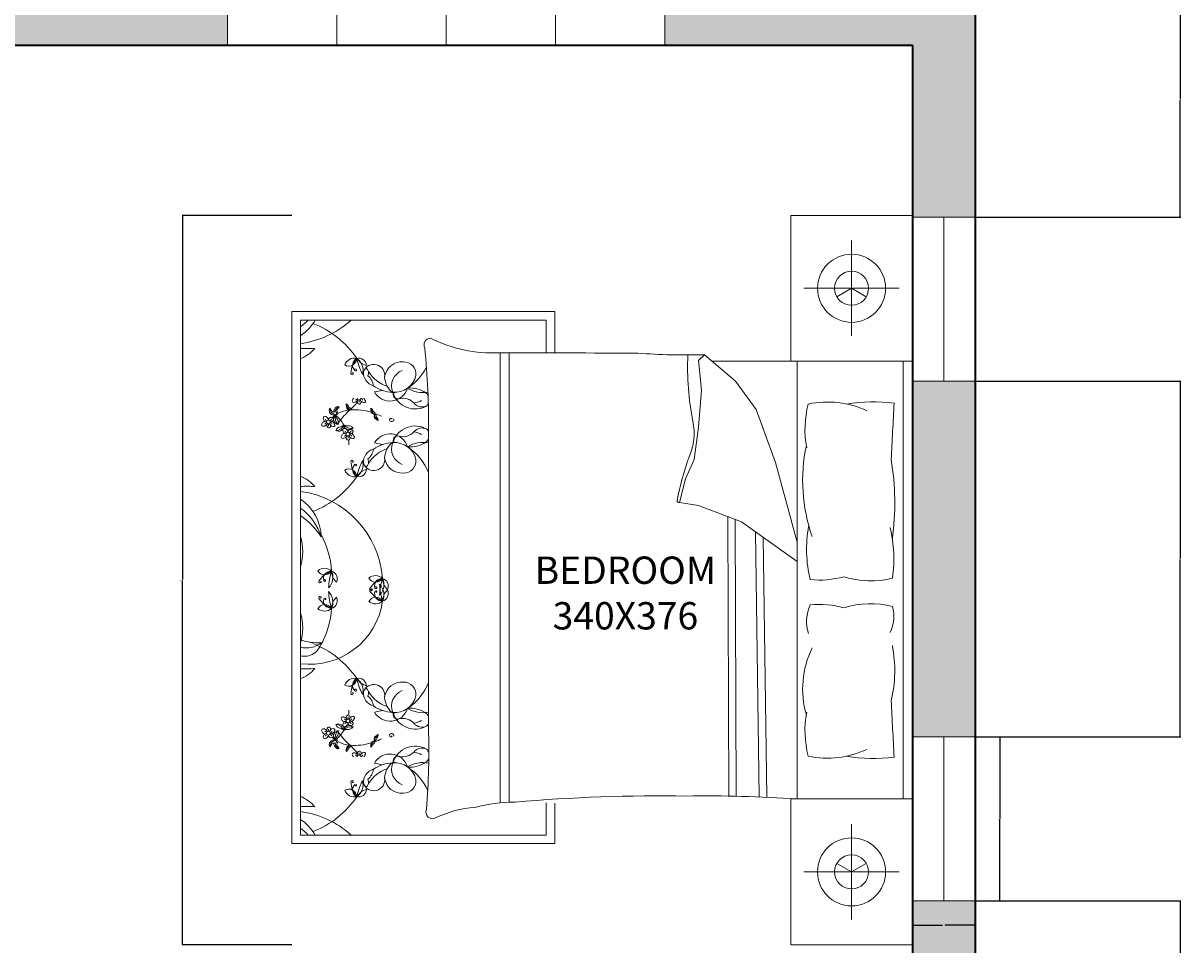
# Model space of a CAD drawing. Units: centimetres. Extents: x 2178 to 3635, y 1064 to 2635.
# Tile 8 of 9: x 3211 to 3635, y 1974 to 2312. Entities that reach past the tile are written whole.
import ezdxf

# ---------------------------------------------------------------- set-up
doc = ezdxf.new("R2010")
doc.units = ezdxf.units.CM
for name, color, linetype, lineweight in [('A-ANNO-DIMS', 2, 'Continuous', 18), ('A-AREA-IDEN', 7, 'Continuous', 18), ('A-FURN', 42, 'Continuous', 18), ('A-GLAZ', 4, 'Continuous', 18), ('A-WALL', 7, 'Continuous', 35)]:
    doc.layers.add(name, color=color, linetype=linetype, lineweight=lineweight)
doc.layers.add('A-WALL-PATT', color=18, linetype='Continuous', lineweight=13, true_color=0x000000)
doc.styles.get("Standard").update_dxf_attribs({"font": 'arial.ttf'})
doc.dimstyles.get("Standard").update_dxf_attribs({"dimtxt": 0.18, "dimasz": 0.18, "dimexe": 0.18, "dimexo": 0.0625, "dimgap": 0.09, "dimtad": 0, "dimtih": 1, "dimtoh": 1, "dimdec": 4, "dimzin": 0, "dimdsep": 46, "dimtxsty": 'Standard', "dimcen": 0.09, "dimadec": 0, "dimazin": 0, "dimtfac": 1, "dimtdec": 4, "dimtofl": 0, "dimtmove": 0, "dimatfit": 3, "dimfxl": 1, "dimtolj": 1, "dimtzin": 0, "dimarcsym": 0})

# ---------------------------------------------------------------- blocks, each defined once
blk = doc.blocks.new('bed')
for p, q in [((2798.77, 2937.13), (3098.77, 2937.13)), ((2858.77, 2937.13), (2858.77, 2854.79)), ((3038.77, 2933.28), (2858.77, 2933.28)), ((2828.77, 2892.53), (2828.77, 2931.73)), ((3068.77, 2892.53), (3068.77, 2931.73)), ((2848.37, 2912.13), (2809.17, 2912.13)), ((3049.17, 2912.13), (3088.37, 2912.13)), ((2858.77, 2889.72), (3038.77, 2889.72)), ((2900.44, 2880.8), (2933.16, 2889.72)), ((2941.19, 2889.72), (2924.75, 2866.84)), ((2878.57, 2872.91), (2900.44, 2880.8)), ((3037.97, 2877.26), (2931.16, 2875.76)), ((2867.02, 2864.41), (2878.57, 2872.91)), ((3037.85, 2874.18), (2928.92, 2872.64)), ((2924.75, 2866.84), (2918.06, 2849.23)), ((2856.09, 2851.66), (2867.02, 2864.41)), ((3037.71, 2861.65), (2922.6, 2861.18)), ((3037.69, 2864.73), (2923.78, 2864.28)), ((2858.52, 2849.23), (2856.09, 2851.66)), ((2870.67, 2850.44), (2858.52, 2849.23)), ((2885.86, 2849.23), (2870.67, 2850.44)), ((2899.23, 2847.41), (2885.86, 2849.23)), ((2907.13, 2843.76), (2899.23, 2847.41)), ((2918.06, 2849.23), (2916.85, 2841.33)), ((2916.85, 2841.33), (2907.13, 2843.76)), ((2838.37, 2790.07), (2855.34, 2790.07)), ((2838.37, 2682), (2838.37, 2790.07)), ((3040.44, 2790.07), (3057.08, 2790.07)), ((3057.08, 2790.07), (3057.08, 2682)), ((2855.33, 2786.59), (2841.85, 2786.59)), ((2841.85, 2786.59), (2841.85, 2685.48)), ((3053.6, 2786.59), (3040.38, 2786.59)), ((3053.6, 2685.48), (3053.6, 2786.59)), ((3040.13, 2771.36), (2855.32, 2771.36)), ((3040.42, 2767.62), (2855.31, 2767.62)), ((3009.67, 2738.15), (2887.87, 2738.15)), ((2871.41, 2715.89), (2870.75, 2719.28)), ((2892.38, 2715.89), (2893.04, 2719.28)), ((3003.07, 2715.89), (3002.41, 2719.28)), ((3024.04, 2715.89), (3024.7, 2719.28)), ((2841.85, 2685.48), (3053.6, 2685.48)), ((3057.08, 2682), (2838.37, 2682))]:
    blk.add_line(p, q)
for points in [[(2858.77, 2887.13), (2798.77, 2887.13), (2798.77, 2937.13)], [(3038.77, 2937.13), (3038.77, 2887.13), (3098.77, 2887.13), (3098.77, 2937.13)], [(2828.77, 2912.13), (2832.27, 2918.19)], [(3068.77, 2912.13), (3065.27, 2918.19)], [(2828.77, 2912.13), (2832.27, 2906.07)], [(3068.77, 2912.13), (3065.27, 2906.07)]]:
    blk.add_lwpolyline(points)
for points in [[(2876, 2929.65, 0.074897), (2876.37, 2910.06, -0.472817)], [(2947.37, 2908.96, 0.14099), (2947.97, 2928.95, 0.235245)], [(2960.18, 2908.96, -0.14099), (2959.58, 2928.95, -0.235245)], [(3021.54, 2929.65, -0.074897), (3021.18, 2910.06, 0.472817)], [(2855.46, 2824.19, 0.001242), (2855.31, 2767.26, -0.127202), (2849.3, 2738.9)], [(3040.05, 2773.72, 0.056112), (3042.23, 2757.21, 0.095341), (3046.45, 2741.32)]]:
    blk.add_lwpolyline(points, format="xyb")
for centre, radius in [((2828.77, 2912.13), 14), ((3068.77, 2912.13), 14), ((2828.77, 2912.13), 7), ((3068.77, 2912.13), 7), ((2888.74, 2705.02), 0.764), ((3006.71, 2705.02), 0.764), ((2883.74, 2696.97), 0.764), ((3011.71, 2696.97), 0.764)]:
    blk.add_circle(centre, radius)
for centre, radius, start, end in [((3041.36, 5784.66), 2859.79, 266.68521, 267.14978), ((2917.11, 2821.09), 108.8, 82.2196, 99.497), ((2940.09, 2876.08), 53.46, 81.5249, 103.96), ((2963.69, 2914.69), 14.84, 63.3437, 106.1026), ((2985.93, 2877.16), 52.74, 76.3427, 101.1841), ((2856.18, 5784.66), 2859.79, 272.85022, 273.31479), ((2914.22, 2902.19), 38.67, 155.1316, 191.7583), ((2983.32, 2902.19), 38.67, 348.2417, 24.8684), ((2912, 2898.93), 36.76, 354.0129, 15.8293), ((2995.54, 2898.93), 36.76, 164.1707, 185.9871), ((2907.87, 2961.74), 69.73, 258.0397, 289.2615), ((2936.1, 2946.52), 52.9, 259.8617, 283.6238), ((2965.7, 2909.52), 15.9, 245.0183, 288.5407), ((2993.49, 2930.2), 38.19, 243.8761, 286.1746), ((2886.7, 2933.16), 40.2, 255.1039, 281.0369), ((3010.84, 2933.16), 40.2, 258.9631, 284.8961), ((3576.57, 2853.06), 539.05, 176.1, 180.9282), ((2581.02, 2844.2), 275.17, 355.8294, 1.553), ((2888.28, 2822.94), 24.42, 66.2616, 101.3392), ((2861.22, 2957.89), 113.22, 267.4519, 281.3392), ((2937.68, 2954.7), 116.34, 250.1194, 259.3383), ((3740.68, 2833.46), 703.17, 179.11454, 184.87351), ((2916.17, 2841.09), 0.724, 268.8623, 19.7536), ((2852.06, 2739.09), 2.77, 183.98, 297.3412), ((2884.29, 2425.86), 312.3, 89.3433, 95.6887), ((2859.22, 2735.93), 12.43, 328.8218, 9.1554), ((2874.61, 2734.83), 3.61, 120.0293, 142.325), ((2874.61, 2734.83), 3.61, 44.4517, 63.558), ((2889.17, 2734.83), 3.61, 113.229, 135.5483), ((2889.17, 2734.83), 3.61, 37.675, 66.7144), ((2904.56, 2735.93), 12.43, 169.7133, 211.1782), ((2912.89, 2717.02), 22.71, 111.4941, 146.3329), ((2982.56, 2717.02), 22.71, 33.6671, 68.5059), ((2990.89, 2735.93), 12.43, 328.8218, 10.2867), ((3006.28, 2734.83), 3.61, 113.2856, 142.325), ((3006.28, 2734.83), 3.61, 44.4517, 66.7144), ((3018.86, 2446.37), 291.92, 85.2402, 91.8035), ((3020.84, 2734.83), 3.61, 106.6343, 135.5483), ((3020.84, 2734.83), 3.61, 37.675, 72.5814), ((3036.23, 2735.93), 12.43, 169.249, 211.1782), ((3044.56, 2717.02), 22.71, 113.6453, 146.3329), ((3044.17, 2739.79), 2.73, 246.5219, 33.8264), ((2864.12, 2727.92), 5.07, 84.4856, 181.0538), ((2850.89, 2717.02), 22.71, 33.6671, 63.2997), ((2862.56, 2724.18), 9.02, 355.2933, 76.921), ((2881.32, 2730.53), 11.57, 145.785, 184.7304), ((2868.85, 2732.7), 9.56, 289.2822, 29.1751), ((2867.4, 2730.97), 8.62, 7.436, 29.9149), ((2873.09, 2735.54), 4.49, 311.5653, 23.8354), ((2894.94, 2732.7), 9.56, 150.8249, 250.7178), ((2890.7, 2735.54), 4.49, 156.1646, 228.4347), ((2896.38, 2730.97), 8.62, 150.0851, 172.564), ((2882.46, 2730.53), 11.57, 355.2696, 34.215), ((2901.22, 2724.18), 9.02, 103.079, 184.7067), ((2899.66, 2727.92), 5.07, 358.9462, 95.5144), ((2995.79, 2727.92), 5.07, 84.4856, 181.0538), ((2994.23, 2724.18), 9.02, 355.2933, 76.921), ((3012.99, 2730.53), 11.57, 145.785, 184.7304), ((3000.51, 2732.7), 9.56, 289.2822, 29.1751), ((2999.07, 2730.97), 8.62, 7.436, 29.9149), ((3004.75, 2735.54), 4.49, 311.5653, 23.8354), ((3026.6, 2732.7), 9.56, 150.8249, 250.7178), ((3022.36, 2735.54), 4.49, 156.1646, 228.4347), ((3028.05, 2730.97), 8.62, 150.0851, 172.564), ((3014.13, 2730.53), 11.57, 355.2696, 34.215), ((3032.89, 2724.18), 9.02, 103.079, 184.7067), ((3031.33, 2727.92), 5.07, 358.9462, 95.5144), ((2867.69, 2722.36), 7.46, 299.9085, 73.1337), ((2880.15, 2727.58), 6.15, 131.5653, 195.1471), ((2883.64, 2727.58), 6.15, 344.8529, 48.4347), ((2896.09, 2722.36), 7.46, 106.8663, 240.0915), ((2999.36, 2722.36), 7.46, 299.9085, 73.1337), ((3011.81, 2727.58), 6.15, 131.5653, 195.1471), ((3015.3, 2727.58), 6.15, 344.8529, 48.4347), ((3027.76, 2722.36), 7.46, 106.8663, 240.0915), ((2866.2, 2727.2), 7.17, 174.9449, 262.8857), ((2869.01, 2729.92), 6.96, 201.5819, 291.4221), ((2864.95, 2728.79), 8.71, 272.3591, 324.0401), ((2855.49, 2724.42), 16.1, 326.2883, 356.5076), ((2881.32, 2730.53), 11.57, 212.7011, 216.3445), ((2872.41, 2725.49), 1.86, 257.3041, 15.1471), ((2882.69, 2723.02), 0.94, 280.4384, 100.4136), ((2891.37, 2725.49), 1.86, 164.8529, 282.6959), ((2882.46, 2730.53), 11.57, 323.6555, 327.2989), ((2898.83, 2728.79), 8.71, 215.9599, 267.6409), ((2894.77, 2729.92), 6.96, 248.5779, 338.4181), ((2908.3, 2724.42), 16.1, 183.4924, 213.7117), ((2897.59, 2727.2), 7.17, 277.1143, 5.0551), ((2997.86, 2727.2), 7.17, 174.9449, 262.8857), ((3000.68, 2729.92), 6.96, 201.5819, 291.4221), ((2996.62, 2728.79), 8.71, 272.3591, 324.0401), ((2987.15, 2724.42), 16.1, 326.2883, 356.5076), ((3012.99, 2730.53), 11.57, 212.7011, 216.3445), ((3004.08, 2725.49), 1.86, 257.3041, 15.1471), ((3012.76, 2723.02), 0.94, 79.5864, 259.5616), ((3023.04, 2725.49), 1.86, 164.8529, 282.6959), ((3014.13, 2730.53), 11.57, 323.6555, 327.2989), ((3030.5, 2728.79), 8.71, 215.9599, 267.6409), ((3026.44, 2729.92), 6.96, 248.5779, 338.4181), ((3039.96, 2724.42), 16.1, 183.4924, 213.7117), ((3029.25, 2727.2), 7.17, 277.1143, 5.0551), ((2864.55, 2715.65), 4.5, 80.264, 250.8688), ((2855.62, 2725.56), 14.16, 301.2614, 341.7045), ((2903.55, 2707.57), 24.85, 153.0032, 159.8941), ((2882.75, 2722.67), 0.578, 102.7051, 280.4384), ((2908.16, 2725.56), 14.16, 198.2955, 238.7386), ((2899.24, 2715.65), 4.5, 289.1312, 99.736), ((2951.1, 2680.2), 39.18, 94.4623, 172.255), ((2951.27, 2716.33), 4.34, 137.7873, 219.1145), ((2946.34, 2716.47), 3.27, 298.5391, 58.3627), ((2951.26, 2719.13), 3.2, 177.7585, 283.852), ((2951.17, 2718.35), 3.25, 63.0274, 163.8037), ((2947.89, 2725.94), 6.69, 271.4585, 315.3727), ((2950.61, 2713.61), 6.19, 45.5411, 114.3101), ((2956.25, 2745.4), 27.41, 252.593, 267.2582), ((2957.43, 2722.47), 9.91, 198.9159, 238.011), ((2954.84, 2713.61), 6.19, 65.6899, 134.4589), ((2949.2, 2745.4), 27.41, 272.7418, 287.407), ((2954.28, 2718.35), 3.25, 16.1963, 116.9726), ((2957.56, 2725.94), 6.69, 224.6273, 268.5415), ((2948.02, 2722.47), 9.91, 301.989, 341.0841), ((2954.19, 2719.13), 3.2, 256.148, 2.2415), ((2959.11, 2716.47), 3.27, 121.6373, 241.4609), ((2954.18, 2716.33), 4.34, 320.8855, 42.2127), ((2953.08, 2689.24), 30.32, 352.8636, 81.8197), ((2996.21, 2715.65), 4.5, 80.264, 250.8688), ((2987.29, 2725.56), 14.16, 301.2614, 341.7045), ((3012.7, 2722.67), 0.578, 259.5616, 77.2949), ((2991.9, 2707.57), 24.85, 20.1059, 26.9968), ((3039.83, 2725.56), 14.16, 198.2955, 238.7386), ((3030.9, 2715.65), 4.5, 289.1312, 99.736), ((2863.47, 2717), 5.62, 265.969, 344.3045), ((2869.52, 2709.53), 5.99, 96.1662, 141.5825), ((2879.44, 2713.73), 1.58, 101.3256, 154.4621), ((2877.17, 2719.07), 4.74, 280.2588, 300.656), ((2878.27, 2722.86), 8.46, 268.3264, 277.1302), ((2903.55, 2707.57), 24.85, 163.5842, 183.8277), ((2876.15, 2719.06), 4.82, 308.2101, 316.3071), ((2879.11, 2715.89), 1.44, 278.3432, 4.2869), ((2878.31, 2717.16), 2.51, 300.656, 332.6341), ((2880.2, 2715.5), 0.611, 55.7657, 157.4417), ((2881.15, 2716.07), 0.611, 84.3784, 186.0543), ((2880.58, 2718.52), 2.51, 269.1859, 301.164), ((2881.32, 2717.22), 1.44, 237.5332, 323.4768), ((2879.92, 2721.32), 4.82, 285.5129, 293.6099), ((2883.07, 2715.9), 1.58, 87.3579, 140.4944), ((2879.43, 2720.42), 4.74, 301.164, 321.5612), ((2875.57, 2721.25), 8.46, 324.6898, 333.4936), ((2894.26, 2709.53), 5.99, 38.4175, 83.8338), ((2900.32, 2717), 5.62, 195.6955, 274.031), ((2951.92, 2716.43), 0.424, 283.852, 219.9245), ((2952.44, 2714.47), 0.487, 238.011, 71.5592), ((2952.52, 2714.71), 0.236, 71.5592, 188.0167), ((2953.01, 2714.47), 0.487, 108.4408, 301.989), ((2952.93, 2714.71), 0.236, 351.9833, 108.4408), ((2953.49, 2716.59), 0.255, 320.1909, 256.0209), ((2995.13, 2717), 5.62, 265.969, 344.3045), ((3001.19, 2709.53), 5.99, 96.1662, 141.5825), ((3012.38, 2715.9), 1.58, 39.5056, 92.6421), ((3016.02, 2720.42), 4.74, 218.4388, 238.836), ((3019.88, 2721.25), 8.46, 206.5064, 215.3102), ((3014.13, 2717.22), 1.44, 216.5232, 302.4668), ((3014.87, 2718.52), 2.51, 238.836, 270.8141), ((3015.53, 2721.32), 4.82, 246.3901, 254.4871), ((3014.3, 2716.07), 0.611, 353.9457, 95.6216), ((3016.34, 2715.89), 1.44, 175.7131, 261.6568), ((3015.25, 2715.5), 0.611, 22.5583, 124.2343), ((3017.14, 2717.16), 2.51, 207.3659, 239.344), ((2991.9, 2707.57), 24.85, 356.1723, 16.4158), ((3019.3, 2719.06), 4.82, 223.6929, 231.7899), ((3018.28, 2719.07), 4.74, 239.344, 259.7412), ((3017.18, 2722.86), 8.46, 262.8698, 271.6736), ((3016.01, 2713.73), 1.58, 25.5379, 78.6744), ((3031.98, 2717), 5.62, 195.6955, 274.031), ((3025.93, 2709.53), 5.99, 38.4175, 83.8338), ((2860.73, 2709.42), 3.25, 92.9516, 193.728), ((2854.09, 2714.37), 6.69, 301.3827, 345.2969), ((2862.6, 2705.03), 6.19, 75.4653, 144.2343), ((2851.64, 2735.41), 27.41, 282.5173, 297.1824), ((2863.62, 2710.77), 2.76, 63.9755, 143.2681), ((2874.99, 2710.74), 1.27, 101.5637, 142.6358), ((2873.93, 2709.56), 0.764, 273.2768, 86.7232), ((2874.82, 2710.28), 0.73, 91.1081, 181.8675), ((2875.59, 2708.82), 1.58, 80.3487, 133.6538), ((2875.31, 2710.12), 1.25, 229.7889, 317.6792), ((2873.96, 2711.74), 1.84, 288.7263, 352.5032), ((2873.9, 2707.47), 1.78, 355.053, 68.3618), ((2875.3, 2707.17), 2.5, 83.0852, 105.7171), ((2875.21, 2711.65), 0.59, 345.2356, 144.9248), ((2875.75, 2709.72), 0.658, 317.6792, 80.3487), ((2900.16, 2710.77), 2.76, 36.7319, 116.0245), ((2901.18, 2705.03), 6.19, 35.7657, 104.5347), ((2912.15, 2735.41), 27.41, 242.8176, 257.4827), ((2903.05, 2709.42), 3.25, 346.272, 87.0484), ((2909.69, 2714.37), 6.69, 194.7031, 238.6173), ((2992.4, 2709.42), 3.25, 92.9516, 193.728), ((2985.76, 2714.37), 6.69, 301.3827, 345.2969), ((2994.27, 2705.03), 6.19, 75.4653, 144.2343), ((2983.3, 2735.41), 27.41, 282.5173, 297.1824), ((2995.29, 2710.77), 2.76, 63.9755, 143.2681), ((3019.7, 2709.72), 0.658, 99.6513, 222.3208), ((3020.14, 2710.12), 1.25, 222.3208, 310.2111), ((3019.86, 2708.82), 1.58, 46.3462, 99.6513), ((3020.24, 2711.65), 0.59, 35.0752, 194.7644), ((3021.49, 2711.74), 1.84, 187.4968, 251.2737), ((3021.55, 2707.47), 1.78, 111.6382, 184.947), ((3020.15, 2707.17), 2.5, 74.2829, 96.9148), ((3020.63, 2710.28), 0.73, 358.1325, 88.8919), ((3020.46, 2710.74), 1.27, 37.3642, 78.4363), ((3021.52, 2709.56), 0.764, 93.2768, 266.7232), ((3031.83, 2710.77), 2.76, 36.7319, 116.0245), ((3032.85, 2705.03), 6.19, 35.7657, 104.5347), ((3043.81, 2735.41), 27.41, 242.8176, 257.4827), ((3041.36, 2714.37), 6.69, 194.7031, 238.6173), ((3034.72, 2709.42), 3.25, 346.272, 87.0484), ((2812.68, 2680.2), 39.18, 7.745, 41.8856), ((2879.7, 2676.32), 39.18, 124.3865, 158.5908), ((2861.82, 2707.73), 4.34, 167.7115, 249.0387), ((2857.48, 2705.38), 3.27, 328.4633, 88.2869), ((2864.1, 2716.11), 9.91, 228.8402, 267.9352), ((2860.42, 2710.14), 3.2, 207.6827, 313.7762), ((2862.34, 2708.13), 0.424, 313.7762, 249.7183), ((2863.71, 2706.94), 0.236, 101.4834, 217.9409), ((2863.76, 2706.7), 0.487, 267.9352, 101.4834), ((2874.97, 2708.15), 1.26, 217.7621, 259.0403), ((2876.33, 2709.83), 2.32, 203.4276, 227.6104), ((2875.09, 2707.37), 0.586, 232.4737, 355.053), ((2857.98, 2686.43), 28.48, 43.1541, 52.0459), ((2877.65, 2703.63), 1.58, 101.3256, 154.4621), ((2875.39, 2708.98), 4.74, 280.2588, 300.656), ((2876.48, 2712.77), 8.46, 268.3264, 277.1302), ((2874.36, 2708.97), 4.82, 308.2101, 316.3071), ((2877.32, 2705.8), 1.44, 278.3432, 4.2869), ((2876.52, 2707.06), 2.51, 300.656, 332.6341), ((2878.41, 2705.4), 0.611, 55.7657, 157.4417), ((2891.17, 2706.94), 12.46, 184.756, 209.2041), ((2909.1, 2733.46), 40.99, 222.2412, 232.1744), ((2884.75, 2705.38), 2.12, 272.8499, 356.1226), ((2882.89, 2706.16), 3.48, 304.5369, 16.3699), ((2883.26, 2704.56), 2.05, 321.7607, 7.9252), ((2887.73, 2705.18), 2.46, 127.3105, 187.9252), ((2884.34, 2705.45), 2.53, 355.0106, 41.658), ((2888.54, 2702.71), 2.41, 104.7558, 148.0499), ((2887.9, 2706.08), 1.04, 126.1046, 271.4281), ((2887.78, 2706.37), 0.749, 353.7526, 131.7054), ((2887.61, 2704.38), 0.506, 262.906, 7.132), ((2887.08, 2705.48), 1.05, 0.0645, 61.1507), ((2887.33, 2706.37), 1.2, 311.8413, 355.7877), ((2889.8, 2706.2), 1.27, 101.5637, 176.365), ((2889.63, 2705.74), 0.73, 91.1081, 181.8675), ((2891.14, 2705.29), 2.32, 203.4276, 227.6104), ((2890.41, 2704.28), 1.58, 80.3487, 133.6538), ((2890.12, 2705.58), 1.25, 229.7889, 317.6792), ((2888.77, 2707.2), 1.84, 288.7263, 352.5032), ((2888.71, 2702.93), 1.78, 355.053, 68.3618), ((2890.11, 2702.63), 2.5, 83.0852, 105.7171), ((2890.02, 2707.11), 0.59, 345.2356, 144.9248), ((2890.56, 2705.18), 0.658, 317.6792, 80.3487), ((2892.45, 2690.4), 14.94, 87.1071, 94.7585), ((2900.02, 2706.7), 0.487, 78.5166, 272.0648), ((2899.68, 2716.11), 9.91, 272.0648, 311.1598), ((2900.07, 2706.94), 0.236, 322.0591, 78.5166), ((2903.37, 2710.14), 3.2, 226.2238, 332.3173), ((2901.49, 2708.3), 0.255, 290.2667, 226.2271), ((2906.3, 2705.38), 3.27, 91.7131, 211.5367), ((2901.96, 2707.73), 4.34, 290.9613, 12.2885), ((2884.08, 2676.32), 39.18, 21.4092, 55.6135), ((3011.37, 2676.32), 39.18, 124.3865, 158.5908), ((2993.49, 2707.73), 4.34, 167.7115, 249.0387), ((2992.08, 2710.14), 3.2, 207.6827, 313.7762), ((2995.76, 2716.11), 9.91, 228.8402, 267.9352), ((2989.15, 2705.38), 3.27, 328.4633, 88.2869), ((2994.01, 2708.13), 0.424, 313.7762, 249.7183), ((2995.38, 2706.94), 0.236, 101.4834, 217.9409), ((2995.43, 2706.7), 0.487, 267.9352, 101.4834), ((3003, 2690.4), 14.94, 85.2415, 92.8929), ((3004.89, 2705.18), 0.658, 99.6513, 222.3208), ((3005.33, 2705.58), 1.25, 222.3208, 310.2111), ((3005.04, 2704.28), 1.58, 46.3462, 99.6513), ((3005.43, 2707.11), 0.59, 35.0752, 194.7644), ((3006.68, 2707.2), 1.84, 187.4968, 251.2737), ((3006.74, 2702.93), 1.78, 111.6382, 184.947), ((3005.34, 2702.63), 2.5, 74.2829, 96.9148), ((3005.82, 2705.74), 0.73, 358.1325, 88.8919), ((3004.31, 2705.29), 2.32, 312.3896, 336.5724), ((3005.65, 2706.2), 1.27, 3.635, 78.4363), ((3007.67, 2706.37), 0.749, 48.2946, 186.2474), ((3008.12, 2706.37), 1.2, 184.2123, 228.1587), ((3008.37, 2705.48), 1.05, 118.8493, 179.9355), ((3007.84, 2704.38), 0.506, 172.868, 277.094), ((3007.55, 2706.08), 1.04, 268.5719, 53.8954), ((3006.91, 2702.71), 2.41, 31.9501, 75.2442), ((3011.11, 2705.45), 2.53, 138.342, 184.9894), ((3010.7, 2705.38), 2.12, 183.8774, 267.1501), ((3012.56, 2706.16), 3.48, 163.6301, 235.4631), ((3007.72, 2705.18), 2.46, 352.0748, 52.6895), ((3012.19, 2704.56), 2.05, 172.0748, 218.2393), ((2986.35, 2733.46), 40.99, 307.8256, 317.7588), ((3004.28, 2706.94), 12.46, 330.7959, 355.244), ((3037.47, 2686.43), 28.48, 127.9541, 136.8459), ((3017.04, 2705.4), 0.611, 22.5583, 124.2343), ((3018.13, 2705.8), 1.44, 175.7131, 261.6568), ((3018.93, 2707.06), 2.51, 207.3659, 239.344), ((3021.09, 2708.97), 4.82, 223.6929, 231.7899), ((3020.06, 2708.98), 4.74, 239.344, 259.7412), ((3018.97, 2712.77), 8.46, 262.8698, 271.6736), ((3017.8, 2703.63), 1.58, 25.5379, 78.6744), ((3020.36, 2707.37), 0.586, 184.947, 307.5263), ((3019.12, 2709.83), 2.32, 312.3896, 336.5724), ((3020.48, 2708.15), 1.26, 280.9597, 322.2379), ((3031.69, 2706.7), 0.487, 78.5166, 272.0648), ((3031.35, 2716.11), 9.91, 272.0648, 311.1598), ((3031.74, 2706.94), 0.236, 322.0591, 78.5166), ((3035.03, 2710.14), 3.2, 226.2238, 332.3173), ((3033.16, 2708.3), 0.255, 290.2667, 226.2271), ((3037.97, 2705.38), 3.27, 91.7131, 211.5367), ((3033.63, 2707.73), 4.34, 290.9613, 12.2885), ((3015.75, 2676.32), 39.18, 21.4092, 55.6135), ((3082.77, 2680.2), 39.18, 138.1144, 172.255), ((2878.18, 2700.87), 0.853, 146.8636, 236.9021), ((2890.21, 2719.66), 22.32, 235.1882, 238.8844), ((2879.65, 2702.11), 2.31, 199.4799, 267.6828), ((2879.39, 2701.23), 1.99, 212.8155, 277.3992), ((2879.13, 2701.31), 0.883, 238.8844, 314.2646), ((2878.94, 2699.33), 1.99, 280.3057, 17.1958), ((2880.21, 2699.7), 0.666, 19.3605, 201.7548), ((2880.22, 2700.2), 0.666, 311.8703, 134.2646), ((2892.74, 2694.13), 13.31, 153.7819, 158.2913), ((2882.15, 2703.22), 3.48, 247.2305, 319.0635), ((2881, 2702.05), 2.05, 264.4544, 310.6188), ((2891.17, 2706.94), 12.46, 214.0033, 222.4917), ((2882.5, 2701.23), 2.12, 218.3208, 298.8162), ((2892.45, 2690.4), 14.94, 120.544, 139.818), ((2883.94, 2698.62), 2.46, 70.0041, 130.6188), ((2882.35, 2701.62), 2.53, 297.7043, 344.3516), ((2885.03, 2699.06), 0.59, 345.2356, 144.9248), ((2883.69, 2701.61), 2.05, 8.7227, 54.8872), ((2883.8, 2699.97), 3.48, 0.278, 72.111), ((2885.36, 2701.25), 2.12, 20.5253, 88.5375), ((2888.15, 2702.29), 2.46, 188.7227, 249.3375), ((2887.13, 2703.59), 0.757, 148.0499, 225.6268), ((2892.45, 2690.4), 14.94, 113.0501, 113.8477), ((2887.18, 2704.44), 1.51, 247.4086, 351.4386), ((2884.99, 2701.06), 2.53, 334.9899, 21.6373), ((2889.78, 2703.61), 1.26, 151.2196, 259.0403), ((2889.9, 2702.83), 0.586, 232.4737, 355.053), ((2948.18, 2697.36), 3.25, 63.0274, 163.8037), ((2944.89, 2704.96), 6.69, 271.4585, 315.3727), ((2957.27, 2697.36), 3.25, 16.1963, 116.9726), ((2960.56, 2704.96), 6.69, 224.6273, 268.5415), ((3005.55, 2702.83), 0.586, 184.947, 307.5263), ((3005.67, 2703.61), 1.26, 280.9597, 28.7804), ((3008.27, 2704.44), 1.51, 188.5614, 292.5914), ((3010.46, 2701.06), 2.53, 158.3627, 205.0101), ((3010.09, 2701.25), 2.12, 91.4625, 159.4747), ((3011.65, 2699.97), 3.48, 107.889, 179.722), ((3007.3, 2702.29), 2.46, 290.6625, 351.2773), ((3008.32, 2703.59), 0.757, 314.3732, 31.9501), ((3003, 2690.4), 14.94, 66.1523, 66.9499), ((3011.76, 2701.61), 2.05, 125.1128, 171.2773), ((3010.42, 2699.06), 0.59, 35.0752, 194.7644), ((3003, 2690.4), 14.94, 40.182, 59.456), ((3011.51, 2698.62), 2.46, 49.3812, 109.9959), ((3013.3, 2703.22), 3.48, 220.9365, 292.7695), ((3013.1, 2701.62), 2.53, 195.6484, 242.2957), ((3012.95, 2701.23), 2.12, 241.1838, 321.6792), ((3014.45, 2702.05), 2.05, 229.3812, 275.5456), ((3004.28, 2706.94), 12.46, 317.5083, 325.9967), ((3016.51, 2699.33), 1.99, 162.8042, 259.6943), ((3015.23, 2700.2), 0.666, 45.7354, 228.1297), ((3015.24, 2699.7), 0.666, 338.2452, 160.6395), ((3002.71, 2694.13), 13.31, 21.7087, 26.2181), ((3016.32, 2701.31), 0.883, 225.7354, 301.1156), ((3016.06, 2701.23), 1.99, 262.6008, 327.1845), ((3015.8, 2702.11), 2.31, 272.3172, 340.5201), ((3005.24, 2719.66), 22.32, 301.1156, 304.8118), ((3017.27, 2700.87), 0.853, 303.0979, 33.1364), ((2878.23, 2699.91), 2.31, 266.9701, 338.2913), ((2866.06, 2716.39), 22.32, 302.6784, 306.3746), ((2878.82, 2698.08), 0.853, 214.3538, 304.3923), ((2878.77, 2699.13), 0.883, 306.3746, 21.7548), ((2882.14, 2695.53), 0.757, 148.0499, 225.6268), ((2883.54, 2694.66), 2.41, 104.7558, 148.0499), ((2882.19, 2696.38), 1.51, 247.4086, 351.4386), ((2882.9, 2698.03), 1.04, 126.1046, 271.4281), ((2882.78, 2698.31), 0.749, 353.7526, 131.7054), ((2882.61, 2696.32), 0.506, 262.906, 7.132), ((2882.08, 2697.42), 1.05, 0.0645, 61.1507), ((2882.33, 2698.32), 1.2, 311.8413, 355.7877), ((2884.78, 2695.55), 1.26, 151.2196, 259.0403), ((2884.8, 2698.15), 1.27, 101.5637, 176.365), ((2884.63, 2697.69), 0.73, 91.1081, 181.8675), ((2886.15, 2697.23), 2.32, 203.4276, 227.6104), ((2885.41, 2696.22), 1.58, 80.3487, 133.6538), ((2885.13, 2697.53), 1.25, 229.7889, 317.6792), ((2883.78, 2699.15), 1.84, 288.7263, 352.5032), ((2883.72, 2694.88), 1.78, 355.053, 68.3618), ((2885.11, 2694.58), 2.5, 83.0852, 105.7171), ((2884.9, 2694.78), 0.586, 232.4737, 355.053), ((2885.56, 2697.13), 0.658, 317.6792, 80.3487), ((2948.1, 2659.21), 39.18, 94.4623, 117.4146), ((2948.27, 2695.35), 4.34, 137.7873, 219.1145), ((2943.34, 2695.48), 3.27, 298.5391, 58.3627), ((2948.26, 2698.14), 3.2, 177.7585, 283.852), ((2947.61, 2692.63), 6.19, 45.5411, 114.3101), ((2954.43, 2701.48), 9.91, 198.9159, 238.011), ((2953.26, 2724.42), 27.41, 252.593, 267.2582), ((2948.92, 2695.44), 0.424, 283.852, 219.9245), ((2957.84, 2692.63), 6.19, 65.6899, 134.4589), ((2952.19, 2724.42), 27.41, 272.7418, 287.407), ((2956.49, 2695.61), 0.255, 320.1909, 256.0209), ((2951.02, 2701.48), 9.91, 301.989, 341.0841), ((2957.19, 2698.14), 3.2, 256.148, 2.2415), ((2962.11, 2695.48), 3.27, 121.6373, 241.4609), ((2957.18, 2695.35), 4.34, 320.8855, 42.2127), ((2957.35, 2659.21), 39.18, 62.5854, 85.5377), ((3009.89, 2697.13), 0.658, 99.6513, 222.3208), ((3010.32, 2697.53), 1.25, 222.3208, 310.2111), ((3010.04, 2696.22), 1.58, 46.3462, 99.6513), ((3011.67, 2699.15), 1.84, 187.4968, 251.2737), ((3011.73, 2694.88), 1.78, 111.6382, 184.947), ((3010.55, 2694.78), 0.586, 184.947, 307.5263), ((3010.34, 2694.58), 2.5, 74.2829, 96.9148), ((3010.82, 2697.69), 0.73, 358.1325, 88.8919), ((3009.3, 2697.23), 2.32, 312.3896, 336.5724), ((3010.65, 2698.15), 1.27, 3.635, 78.4363), ((3010.67, 2695.55), 1.26, 280.9597, 28.7804), ((3013.26, 2696.38), 1.51, 188.5614, 292.5914), ((3012.67, 2698.31), 0.749, 48.2946, 186.2474), ((3013.12, 2698.32), 1.2, 184.2123, 228.1587), ((3013.37, 2697.42), 1.05, 118.8493, 179.9355), ((3012.84, 2696.32), 0.506, 172.868, 277.094), ((3012.55, 2698.03), 1.04, 268.5719, 53.8954), ((3011.91, 2694.66), 2.41, 31.9501, 75.2442), ((3013.31, 2695.53), 0.757, 314.3732, 31.9501), ((3017.22, 2699.91), 2.31, 201.7087, 273.0299), ((3016.68, 2699.13), 0.883, 158.2452, 233.6254), ((3029.39, 2716.39), 22.32, 233.6254, 237.3216), ((3016.63, 2698.08), 0.853, 235.6077, 325.6462), ((2832.33, 2674.95), 19.09, 33.4617, 60.1116), ((2843.02, 2679.37), 15.93, 22.5547, 48.9546), ((2799.39, 2687.93), 54.2, 357.4081, 3.6519), ((2920.76, 2679.37), 15.93, 131.0454, 157.4453), ((2964.39, 2687.93), 54.2, 176.3481, 182.5919), ((2931.45, 2674.95), 19.09, 91.272, 146.5383), ((2938.32, 2671.39), 23.79, 107.8504, 143.6964), ((2950.82, 2664.7), 35.39, 124.0123, 144.053), ((2949.44, 2693.49), 0.487, 238.011, 71.5592), ((2949.52, 2693.73), 0.236, 71.5592, 188.0167), ((2956.01, 2693.49), 0.487, 108.4408, 301.989), ((2955.93, 2693.73), 0.236, 351.9833, 108.4408), ((2957, 2692.01), 17.54, 338.117, 6.6195), ((2973.09, 2687.13), 7.03, 346.3898, 79.0739), ((2967.81, 2688.1), 8.89, 342.8609, 41.9049), ((2931.06, 2687.93), 54.2, 357.4081, 3.6519), ((2974.69, 2679.37), 15.93, 22.5547, 48.9546), ((3052.43, 2679.37), 15.93, 131.0454, 157.4453), ((3096.06, 2687.93), 54.2, 176.3481, 182.5919), ((3063.12, 2674.95), 19.09, 119.8884, 146.5383), ((2825.46, 2671.39), 23.79, 36.3036, 46.4814), ((2937.15, 2664.88), 21.54, 73.5431, 107.0202), ((2945.68, 2653.78), 31.85, 94.3787, 95.6357), ((2962.46, 2631.95), 56.92, 109.7217, 109.9028), ((2968.3, 2664.88), 21.54, 72.9798, 106.4569), ((2959.77, 2653.78), 31.85, 84.3643, 85.6213), ((2942.99, 2631.95), 56.92, 70.0972, 70.2783), ((3069.99, 2671.39), 23.79, 133.5186, 143.6964)]:
    blk.add_arc(centre, radius, start, end)
blk = doc.blocks.new('WIN-1600-4LT')
for p, q in [((0, 23), (0, 0)), ((40, 23), (40, 0)), ((80, 23), (80, 0)), ((120, 23), (120, 0)), ((160, 23), (160, 0)), ((0, 11.5), (160, 11.5))]:
    blk.add_line(p, q)
blk = doc.blocks.new('WIN-0600')
for p, q in [((0, 60), (23, 60)), ((11.5, 60), (11.5, 0)), ((0, 0), (23, 0))]:
    blk.add_line(p, q)
blk = doc.blocks.new('*D26')
at = {"layer": 'A-ANNO-DIMS', "color": 0, "lineweight": -2, "transparency": 16777216}
for p, q in [((3559.67, 2050.59), (3568.78, 2050.59)), ((3568.6, 2050.41), (3568.6, 2020.77)), ((3568.6, 1990.77), (3568.6, 2020.41)), ((3559.67, 1990.59), (3568.78, 1990.59))]:
    blk.add_line(p, q, dxfattribs=at)
at = {"layer": 'A-ANNO-DIMS', "color": 0, "transparency": 16777216}
for points in [[(3568.57, 2050.41), (3568.63, 2050.41), (3568.6, 2050.59)], [(3568.57, 1990.77), (3568.63, 1990.77), (3568.6, 1990.59)]]:
    blk.add_solid(points, dxfattribs=at)
at = {"layer": 'Defpoints', "color": 0, "transparency": 16777216}
for p in [(3559.6, 2050.59), (3568.6, 2050.59), (3559.6, 1990.59)]:
    blk.add_point(p, dxfattribs=at)
at = {"layer": 'A-ANNO-DIMS', "color": 0, "transparency": 16777216, "insert": (3568.6, 2020.59), "char_height": 0.18, "attachment_point": 5}
blk.add_mtext('\\A1;WIN. 60 TYP.', dxfattribs=at)
blk = doc.blocks.new('*D27')
at = {"layer": 'A-ANNO-DIMS', "color": 0, "lineweight": -2, "transparency": 16777216}
for p, q in [((3536.6, 1990.53), (3536.6, 1981.41)), ((3559.6, 1990.53), (3559.6, 1981.41)), ((3536.78, 1981.59), (3547.58, 1981.59)), ((3559.42, 1981.59), (3548.63, 1981.59))]:
    blk.add_line(p, q, dxfattribs=at)
at = {"layer": 'A-ANNO-DIMS', "color": 0, "transparency": 16777216}
for points in [[(3536.78, 1981.62), (3536.78, 1981.56), (3536.6, 1981.59)], [(3559.42, 1981.62), (3559.42, 1981.56), (3559.6, 1981.59)]]:
    blk.add_solid(points, dxfattribs=at)
at = {"layer": 'Defpoints', "color": 0, "transparency": 16777216}
for p in [(3536.6, 1990.59), (3559.6, 1990.59), (3559.6, 1981.59)]:
    blk.add_point(p, dxfattribs=at)
at = {"layer": 'A-ANNO-DIMS', "color": 0, "transparency": 16777216, "insert": (3548.1, 1981.59), "char_height": 0.18, "attachment_point": 5}
blk.add_mtext('\\A1;23 TYP.', dxfattribs=at)
blk = doc.blocks.new('*D28')
at = {"layer": 'A-ANNO-DIMS', "color": 0, "lineweight": -2, "transparency": 16777216}
for p, q in [((3309.61, 2241.29), (3269.47, 2241.29)), ((3269.65, 2241.11), (3269.65, 2108.05)), ((3269.65, 1974.63), (3269.65, 2107.68)), ((3309.61, 1974.45), (3269.47, 1974.45))]:
    blk.add_line(p, q, dxfattribs=at)
at = {"layer": 'A-ANNO-DIMS', "color": 0, "transparency": 16777216}
for points in [[(3269.62, 2241.11), (3269.68, 2241.11), (3269.65, 2241.29)], [(3269.62, 1974.63), (3269.68, 1974.63), (3269.65, 1974.45)]]:
    blk.add_solid(points, dxfattribs=at)
at = {"layer": 'Defpoints', "color": 0, "transparency": 16777216}
for p in [(3309.68, 2241.29), (3269.65, 1974.45), (3309.68, 1974.45)]:
    blk.add_point(p, dxfattribs=at)
at = {"layer": 'A-ANNO-DIMS', "color": 0, "transparency": 16777216, "insert": (3269.65, 2107.87), "char_height": 0.18, "attachment_point": 5}
blk.add_mtext('\\A1;BED GROUP 267 TYP.', dxfattribs=at)
blk = doc.blocks.new('*D54')
at = {"layer": 'A-ANNO-DIMS', "color": 0, "lineweight": -2, "transparency": 16777216}
for p, q in [((3559.67, 2326.59), (3634.78, 2326.59)), ((3634.6, 2326.41), (3634.6, 2283.77)), ((3634.6, 2240.77), (3634.6, 2283.41)), ((3559.67, 2240.59), (3634.78, 2240.59))]:
    blk.add_line(p, q, dxfattribs=at)
at = {"layer": 'A-ANNO-DIMS', "color": 0, "transparency": 16777216}
for points in [[(3634.57, 2326.41), (3634.63, 2326.41), (3634.6, 2326.59)], [(3634.57, 2240.77), (3634.63, 2240.77), (3634.6, 2240.59)]]:
    blk.add_solid(points, dxfattribs=at)
at = {"layer": 'Defpoints', "color": 0, "transparency": 16777216}
for p in [(3559.6, 2326.59), (3634.6, 2326.59), (3559.6, 2240.59)]:
    blk.add_point(p, dxfattribs=at)
at = {"layer": 'A-ANNO-DIMS', "color": 0, "transparency": 16777216, "insert": (3634.6, 2283.59), "char_height": 0.18, "attachment_point": 5}
blk.add_mtext('\\A1;86', dxfattribs=at)
blk = doc.blocks.new('*D55')
at = {"layer": 'A-ANNO-DIMS', "color": 0, "lineweight": -2, "transparency": 16777216}
for p, q in [((3559.67, 2180.59), (3634.78, 2180.59)), ((3634.6, 2180.41), (3634.6, 2115.77)), ((3634.6, 2050.77), (3634.6, 2115.41)), ((3559.67, 2050.59), (3634.78, 2050.59))]:
    blk.add_line(p, q, dxfattribs=at)
at = {"layer": 'A-ANNO-DIMS', "color": 0, "transparency": 16777216}
for points in [[(3634.57, 2180.41), (3634.63, 2180.41), (3634.6, 2180.59)], [(3634.57, 2050.77), (3634.63, 2050.77), (3634.6, 2050.59)]]:
    blk.add_solid(points, dxfattribs=at)
at = {"layer": 'Defpoints', "color": 0, "transparency": 16777216}
for p in [(3559.6, 2180.59), (3634.6, 2180.59), (3559.6, 2050.59)]:
    blk.add_point(p, dxfattribs=at)
at = {"layer": 'A-ANNO-DIMS', "color": 0, "transparency": 16777216, "insert": (3634.6, 2115.59), "char_height": 0.18, "attachment_point": 5}
blk.add_mtext('\\A1;130', dxfattribs=at)
blk = doc.blocks.new('*D56')
at = {"layer": 'A-ANNO-DIMS', "color": 0, "lineweight": -2, "transparency": 16777216}
for p, q in [((3559.67, 1990.59), (3634.78, 1990.59)), ((3634.6, 1990.41), (3634.6, 1959.27)), ((3634.6, 1927.77), (3634.6, 1958.91)), ((3536.67, 1927.59), (3634.78, 1927.59))]:
    blk.add_line(p, q, dxfattribs=at)
at = {"layer": 'A-ANNO-DIMS', "color": 0, "transparency": 16777216}
for points in [[(3634.57, 1990.41), (3634.63, 1990.41), (3634.6, 1990.59)], [(3634.57, 1927.77), (3634.63, 1927.77), (3634.6, 1927.59)]]:
    blk.add_solid(points, dxfattribs=at)
at = {"layer": 'Defpoints', "color": 0, "transparency": 16777216}
for p in [(3559.6, 1990.59), (3634.6, 1990.59), (3536.6, 1927.59)]:
    blk.add_point(p, dxfattribs=at)
at = {"layer": 'A-ANNO-DIMS', "color": 0, "transparency": 16777216, "insert": (3634.6, 1959.09), "char_height": 0.18, "attachment_point": 5}
blk.add_mtext('\\A1;63', dxfattribs=at)

msp = doc.modelspace()

# ---------------------------------------------------------------- hatches: boundary and pattern name
at = {"layer": 'A-WALL-PATT'}
h = msp.add_hatch(color=256, dxfattribs=at)
h.dxf.hatch_style = 1
h.paths.add_polyline_path([(2276.605, 2499.59), (2253.605, 2499.59), (2253.605, 2476.59), (2276.605, 2476.59)])
h.paths.add_polyline_path([(2411.605, 2350.59), (2253.605, 2350.59), (2253.605, 2327.59), (2411.605, 2327.59)])
h.paths.add_polyline_path([(2276.605, 2252.59), (2253.605, 2252.59), (2253.605, 2020.59), (2276.605, 2020.59), (2276.605, 2093.59), (2561.605, 2093.59), (2561.605, 2116.59), (2276.605, 2116.59)])
h.paths.add_polyline_path([(2659.605, 1787.59), (2610.616, 1787.59), (2276.605, 1787.59), (2276.605, 1860.59), (2253.605, 1860.59), (2253.605, 1732.09), (2276.605, 1732.09), (2276.605, 1764.59), (2516.605, 1764.59), (2516.605, 1699.59), (2539.605, 1699.59), (2539.605, 1764.59), (2659.605, 1764.59)])
h.paths.add_polyline_path([(2539.605, 1624.59), (2276.605, 1624.59), (2276.605, 1657.09), (2253.605, 1657.09), (2253.605, 1561.59), (2276.605, 1561.59), (2276.605, 1601.59), (2539.605, 1601.59)])
h.paths.add_polyline_path([(2276.605, 1501.59), (2253.605, 1501.59), (2253.605, 1371.59), (2276.605, 1371.59)])
h.paths.add_polyline_path([(2376.605, 1271.59), (2276.605, 1271.59), (2276.605, 1311.59), (2253.605, 1311.59), (2253.605, 1248.59), (2376.605, 1248.59)])
h.paths.add_polyline_path([(2636.605, 1271.59), (2536.605, 1271.59), (2536.605, 1248.59), (2636.605, 1248.59)])
h.paths.add_polyline_path([(2659.605, 1600.59), (2919.605, 1600.59), (2919.605, 1623.59), (2636.605, 1623.59), (2636.605, 1188.59), (2659.605, 1188.59)])
h.paths.add_polyline_path([(2939.605, 1211.59), (2759.605, 1211.59), (2759.605, 1188.59), (2939.605, 1188.59)])
h.paths.add_polyline_path([(3062.605, 1288.59), (3039.605, 1288.59), (3039.605, 1188.59), (3062.605, 1188.59)])
h.paths.add_polyline_path([(3372.605, 1248.59), (3062.605, 1248.59), (3062.605, 1218.59), (3372.605, 1218.59)])
h.paths.add_polyline_path([(3395.605, 1271.59), (3372.605, 1271.59), (3372.605, 1248.59), (3395.605, 1248.59)])
h.paths.add_polyline_path([(3559.605, 1271.59), (3536.605, 1271.59), (3536.605, 1248.59), (3559.605, 1248.59)])
h.paths.add_polyline_path([(3559.605, 1623.59), (3536.605, 1623.59), (3536.605, 1600.59), (3559.605, 1600.59)])
h.paths.add_polyline_path([(3395.605, 1623.59), (3162.605, 1623.59), (3162.605, 1600.59), (3395.605, 1600.59)])
h.paths.add_polyline_path([(3395.605, 1411.59), (3277.1, 1411.59), (3277.1, 1388.59), (3395.605, 1388.59)])
h.paths.add_polyline_path([(3157.1, 1411.59), (3062.605, 1411.59), (3062.605, 1623.59), (3039.605, 1623.59), (3039.605, 1388.59), (3157.1, 1388.59)])
h.paths.add_polyline_path([(3559.605, 1797.09), (3536.605, 1797.09), (3536.605, 1764.59), (3316.605, 1764.59), (3316.605, 1927.59), (3293.605, 1927.59), (3293.605, 1741.59), (3372.605, 1741.59), (3395.605, 1741.59), (3559.605, 1741.59)])
h.paths.add_polyline_path([(3559.605, 1990.59), (3536.605, 1990.59), (3536.605, 1974.446), (3536.605, 1927.59), (3391.605, 1927.59), (3391.605, 1904.59), (3536.605, 1904.59), (3536.605, 1872.09), (3559.605, 1872.09)])
h.paths.add_polyline_path([(3559.605, 2180.59), (3536.605, 2180.59), (3536.605, 2050.59), (3559.605, 2050.59)])
h.paths.add_polyline_path([(3559.605, 2326.59), (3446.105, 2326.59), (3446.105, 2303.59), (3536.605, 2303.59), (3536.605, 2240.59), (3559.605, 2240.59)])
h.paths.add_polyline_path([(3286.105, 2326.59), (3195.605, 2326.59), (3195.605, 2499.59), (3082.605, 2499.59), (3082.605, 2476.59), (3172.605, 2476.59), (3172.605, 2116.59), (2809.605, 2116.59), (2809.605, 2093.59), (3172.605, 2093.59), (3172.605, 1904.59), (3195.605, 1904.59), (3195.605, 2303.59), (3286.105, 2303.59)])
h.paths.add_polyline_path([(2832.605, 2236.59), (2659.605, 2236.59), (2659.605, 2476.59), (2697.105, 2476.59), (2697.105, 2499.59), (2636.605, 2499.59), (2636.605, 2093.59), (2699.605, 2093.59), (2699.605, 2116.59), (2659.605, 2116.59), (2659.605, 2213.59), (2832.605, 2213.59)])
h.paths.add_polyline_path([(2832.605, 2476.59), (2922.605, 2476.59), (2922.605, 2499.59), (2772.105, 2499.59), (2772.105, 2476.59), (2809.605, 2476.59), (2809.605, 2311.59), (2832.605, 2311.59)])

# ---------------------------------------------------------------- linework, layer by layer
at = {"layer": 'A-WALL'}
for p, q in [((3559.605, 2326.59), (3559.605, 1188.59)), ((3195.605, 2303.59), (3536.605, 2303.59)), ((3536.605, 2303.59), (3536.605, 1927.59))]:
    msp.add_line(p, q, dxfattribs=at)

# ---------------------------------------------------------------- block references
at = {"layer": 'A-FURN', "xscale": 0.8894661318613604, "yscale": 0.8894661318613604, "zscale": 0.8894661318613604, "rotation": 270}
msp.add_blockref('bed', (924.128, 4730.698), dxfattribs=at)
at = {"layer": 'A-GLAZ'}
for name, p in [('WIN-1600-4LT', (3286.105, 2303.59)), ('WIN-0600', (3536.605, 1990.59))]:
    msp.add_blockref(name, p, dxfattribs=at)
at = {"layer": 'A-GLAZ', "rotation": 180}
msp.add_blockref('WIN-0600', (3559.605, 2240.59), dxfattribs=at)

# ---------------------------------------------------------------- texts
at = {"layer": 'A-AREA-IDEN', "insert": (3375.859, 2116.485), "char_height": 10, "attachment_point": 1}
msp.add_mtext_dynamic_manual_height_columns('\\pxqc;BEDROOM\\P340X376', width=111.5542, gutter_width=12.5, heights=[0], dxfattribs=at)

# ---------------------------------------------------------------- dimensions: what is measured, and where the dimension line sits
at = {"layer": 'A-ANNO-DIMS'}
for base, p1, p2, picture, middle in [((3634.605, 2326.59), (3559.605, 2240.59), (3559.605, 2326.59), '*D54', (3634.605, 2283.59)), ((3634.605, 2180.59), (3559.605, 2050.59), (3559.605, 2180.59), '*D55', (3634.605, 2115.59)), ((3634.605, 1990.59), (3536.605, 1927.59), (3559.605, 1990.59), '*D56', (3634.605, 1959.09))]:
    dim = msp.add_linear_dim(base=base, p1=p1, p2=p2, angle=90, dimstyle='Standard', override={"dimdec": 0, "dimlfac": 1, "dimrnd": 0, "dimzin": 0, "dimdsep": 46, "dimlunit": 2}, dxfattribs=at)
    dim.commit()
    dim.dimension.update_dxf_attribs({"geometry": picture, "text_midpoint": middle})
for base, p1, p2, angle, text, picture, middle in [((3269.649, 1974.446), (3309.675, 2241.286), (3309.675, 1974.446), 270, 'BED GROUP <> TYP.', '*D28', (3269.649, 2107.866)), ((3568.605, 2050.59), (3559.605, 1990.59), (3559.605, 2050.59), 90, 'WIN. <> TYP.', '*D26', (3568.605, 2020.59))]:
    dim = msp.add_linear_dim(base=base, p1=p1, p2=p2, angle=angle, text=text, dimstyle='Standard', override={"dimdec": 0, "dimlfac": 1, "dimrnd": 0, "dimzin": 0, "dimdsep": 46, "dimlunit": 2}, dxfattribs=at)
    dim.commit()
    dim.dimension.update_dxf_attribs({"geometry": picture, "text_midpoint": middle})
dim = msp.add_linear_dim(base=(3559.605, 1981.59), p1=(3536.605, 1990.59), p2=(3559.605, 1990.59), text='<> TYP.', dimstyle='Standard', override={"dimdec": 0, "dimlfac": 1, "dimrnd": 0, "dimzin": 0, "dimdsep": 46, "dimlunit": 2}, dxfattribs=at)
dim.commit()
dim.dimension.update_dxf_attribs({"geometry": '*D27', "text_midpoint": (3548.105, 1981.59)})

doc.saveas('drawing.dxf')
